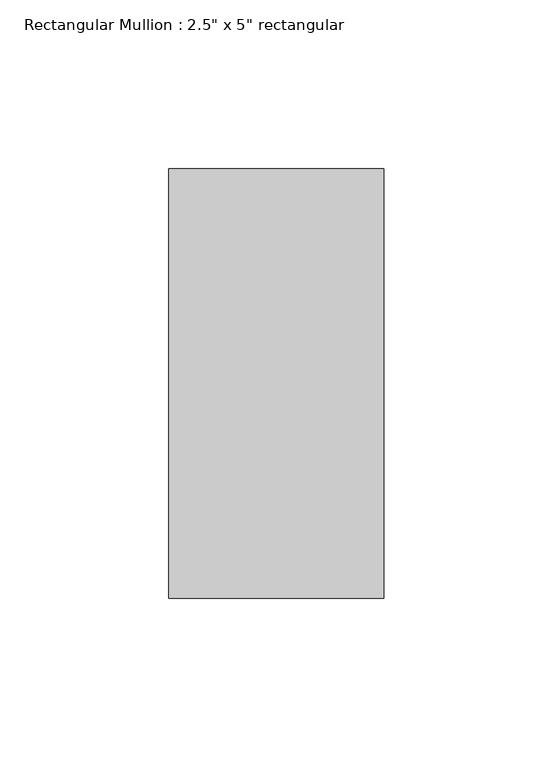
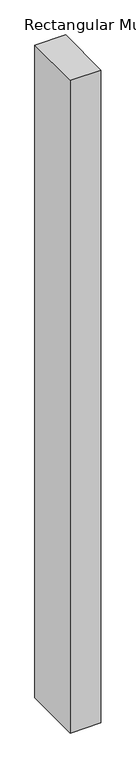
"""IFC4 building model written with IfcOpenShell, lengths in millimetres: member geometry."""

from ifc_helpers import new_model, si_unit, frame, origin, place, context, project, spatial, polyline, outline, extrude, source, transform, mapped, element, save


def member_c6cbf9be(model_context):
    return source(origin(), model_context, "Body", "SweptSolid", [
        extrude(outline(polyline([(0.0, 63.5), (0.0, -63.5), (-63.5, -63.5), (-63.5, 63.5), (0.0, 63.5)])), frame((0.0, 0.0, -1432.9498103), z_axis=(0.0, 0.0, 1.0), x_axis=(1.0, 0.0, 0.0)), (0.0, 0.0, 1.0), 1432.9498103),
    ])


if __name__ == "__main__":
    model = new_model("IFC4")
    model_context = context("Model", 3, world=origin())
    ifc_project = project(units=[si_unit("LENGTHUNIT", "METRE", prefix="MILLI")], contexts=[model_context])
    site = spatial("IfcSite", under=ifc_project)
    building = spatial("IfcBuilding", under=site)
    placement = place(None, origin())
    member_shape = member_c6cbf9be(model_context)
    element("IfcMember", 1, ObjectType="Rectangular Mullion : 2.5\" x 5\" rectangular", at=placement, inside=building, context=model_context, shape_type="MappedRepresentation", body=[
        mapped(member_shape, transform((0.0, 0.0, 0.0), x_axis=(1.0, 0.0, 0.0), y_axis=(0.0, 1.0, 0.0), z_axis=(0.0, 0.0, 1.0))),
    ])
    save(model, "model.ifc")

# Revit data of these elements
# Type "Rectangular Mullion : 2.5\" x 5\" rectangular"
#   built-in parameter 1007304 = 0.416667 (stored number, unit not read)
#   built-in parameter 1007301 = 0.104167 (stored number, unit not read)
#   built-in parameter 1007300 = 0.104167 (stored number, unit not read)
# Element 1 (IfcMember, "Rectangular Mullion : 2.5\" x 5\" rectangular")
#   Materials on its faces: "Aluminum"
# Materials
#   "Aluminum": class "Metal", colour RGB 247 247 247, transparency 0, Description = "Aluminum 6061", Cost = 0
